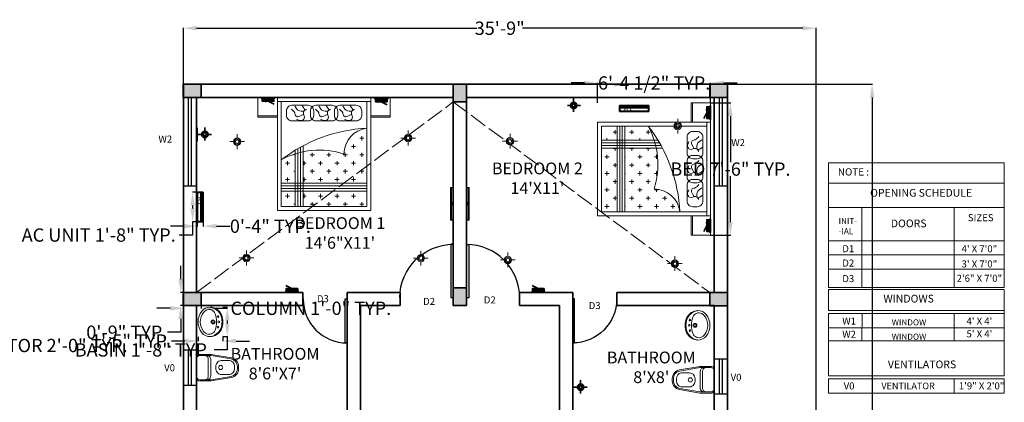
# Model space of a CAD drawing. Units: inches. Extents: x 68 to 1275, y 90 to 1276.
# Tile 6 of 6: x 608 to 1275, y 1017 to 1276. Entities that reach past the tile are written whole.
import ezdxf

# ---------------------------------------------------------------- set-up
doc = ezdxf.new("R2010")
doc.units = ezdxf.units.IN
doc.header["$MEASUREMENT"] = 0
doc.linetypes.add('ACAD_ISO02W100', pattern=[15, 12, -3])
for name, color, linetype, lineweight in [('A -Elec', 6, 'Continuous', 18), ('A-ANNO-SCHD', 8, 'Continuous', 13), ('A-ANNO-TEXT', 7, 'Continuous', 18), ('A-AREA-IDEN', 7, 'Continuous', 18), ('A-FLOR-FIXT', 9, 'Continuous', 18), ('A-FURN', 150, 'Continuous', 5), ('A-WALL', 7, 'Continuous', 35), ('COLUMN', 150, 'Continuous', 35), ('DIM', 2, 'Continuous', 18), ('DOOR', 15, 'Continuous', 25), ('E-EQPM', 1, 'Continuous', 18), ('E-LITE', 6, 'Continuous', 18), ('E-POWR', 1, 'Continuous', 18), ('E-REFR', 8, 'ACAD_ISO02W100', 13), ('Elec', 1, 'Continuous', 35), ('FURN', 163, 'Continuous', 18), ('WINDOW', 17, 'Continuous', 18)]:
    doc.layers.add(name, color=color, linetype=linetype, lineweight=lineweight)
doc.styles.get("Standard").update_dxf_attribs({"font": 'arial.ttf'})
doc.dimstyles.get("Standard").update_dxf_attribs({"dimtxt": 9, "dimasz": 9, "dimexe": 0.18, "dimexo": 0.0625, "dimgap": 0.09, "dimtad": 0, "dimtih": 1, "dimtoh": 1, "dimdec": 1, "dimzin": 0, "dimdsep": 46, "dimlunit": 3, "dimtxsty": 'Standard', "dimcen": 0.09, "dimadec": 0, "dimazin": 0, "dimtfac": 1, "dimtdec": 1, "dimtofl": 0, "dimtmove": 0, "dimatfit": 3, "dimfxl": 1, "dimtolj": 1, "dimtzin": 0, "dimarcsym": 0})

# ---------------------------------------------------------------- blocks, each defined once
blk = doc.blocks.new('*U2')
for p, q in [((0, 0), (0, -6)), ((40, 0), (40, -6))]:
    blk.add_line(p, q)
blk.add_lwpolyline([(0, 0), (0, 40), (1.75, 40), (1.75, 0)], close=True)
blk.add_arc((0, 0), 40, 0, 90)
blk = doc.blocks.new('W')
at = {"layer": 'DOOR'}
for p, q in [((91.84, 414.95), (100.84, 414.95)), ((91.84, 354.95), (91.84, 414.95)), ((95.34, 354.95), (95.34, 414.95)), ((97.34, 354.95), (97.34, 414.95)), ((100.84, 414.95), (100.84, 354.95)), ((100.84, 354.95), (91.84, 354.95))]:
    blk.add_line(p, q, dxfattribs=at)
blk = doc.blocks.new('V')
at = {"layer": 'DOOR'}
for p, q in [((554.81, 674.59), (563.81, 674.59)), ((554.81, 650.59), (554.81, 674.59)), ((558.31, 650.59), (558.31, 674.59)), ((560.31, 650.59), (560.31, 674.59)), ((563.81, 674.59), (563.81, 650.59)), ((563.81, 650.59), (554.81, 650.59))]:
    blk.add_line(p, q, dxfattribs=at)
blk = doc.blocks.new('C')
h = blk.add_hatch(color=256)
h.dxf.hatch_style = 1
h.paths.add_polyline_path([(745.81, 845.98), (745.81, 857.98), (736.81, 857.98), (736.81, 845.98)])
for p, q in [((745.81, 857.98), (736.81, 857.98)), ((736.81, 857.98), (736.81, 845.98)), ((745.81, 845.98), (745.81, 857.98)), ((736.81, 845.98), (745.81, 845.98))]:
    blk.add_line(p, q)
blk = doc.blocks.new('bed 1')
at = {"layer": 'FURN'}
h = blk.add_hatch(dxfattribs=at)
h.set_pattern_fill('CROSS', color=256, style=0)
h.set_pattern_definition([(0, (0, 0), (6.35, 6.35), [3.175, -9.525]), (90, (1.5875, -1.5875), (-6.35, 6.35), [3.175, -9.525])])
h.paths.add_polyline_path([(1334.16, -843.32, 0.37496), (1316.43, -863.27, 0.131129), (1284.95, -861.51), (1284.95, -885.72), (1334.16, -885.72)])
h.paths.add_polyline_path([(1278.95, -863.08, 0.048033), (1268.16, -867.67), (1268.16, -885.72), (1278.95, -885.72)])
h.paths.add_polyline_path([(1278.95, -891.72), (1268.16, -891.72), (1268.16, -903.72), (1278.95, -903.72)])
h.paths.add_polyline_path([(1334.16, -891.72), (1284.95, -891.72), (1284.95, -903.72), (1334.16, -903.72)])
for p, q in [((1265.16, -819.72), (1250.16, -819.72)), ((1250.16, -819.72), (1250.16, -834.72)), ((1337.16, -819.72), (1265.16, -819.72)), ((1265.16, -819.72), (1265.16, -906.72)), ((1337.16, -822.72), (1265.16, -822.72)), ((1268.16, -822.72), (1268.16, -903.72)), ((1334.16, -903.72), (1334.16, -822.72)), ((1337.16, -906.72), (1337.16, -819.72)), ((1337.16, -819.72), (1352.16, -819.72)), ((1352.16, -819.72), (1352.16, -834.72)), ((1250.16, -833.72), (1265.16, -833.72)), ((1352.16, -833.72), (1337.16, -833.72)), ((1250.16, -834.72), (1265.16, -834.72)), ((1352.16, -834.72), (1337.16, -834.72)), ((1284.95, -903.72), (1284.95, -856.89)), ((1278.95, -903.72), (1278.95, -860.29)), ((1280.95, -903.72), (1280.95, -859.11)), ((1282.95, -903.72), (1282.95, -857.98)), ((1334.16, -885.72), (1268.16, -885.72)), ((1334.16, -887.72), (1268.16, -887.72)), ((1334.16, -889.72), (1268.16, -889.72)), ((1334.16, -891.72), (1268.16, -891.72)), ((1265.16, -906.72), (1337.16, -906.72)), ((1268.16, -903.72), (1334.16, -903.72))]:
    blk.add_line(p, q, dxfattribs=at)
for points in [[(1288.91, -837.72), (1276.42, -837.72, -0.414214), (1272.16, -833.47), (1272.16, -829.98, -0.414214), (1276.42, -825.72), (1288.91, -825.72, -0.414214), (1293.16, -829.98), (1293.16, -833.47, -0.414214)], [(1307.41, -837.72), (1294.92, -837.72, -0.414214), (1290.66, -833.47), (1290.66, -829.98, -0.414214), (1294.92, -825.72), (1307.41, -825.72, -0.414214), (1311.66, -829.98), (1311.66, -833.47, -0.414214)], [(1325.91, -837.72), (1313.42, -837.72, -0.414214), (1309.16, -833.47), (1309.16, -829.98, -0.414214), (1313.42, -825.72), (1325.91, -825.72, -0.414214), (1330.16, -829.98), (1330.16, -833.47, -0.414214)], [(1334.16, -843.32, 0.151933), (1268.16, -867.67), (1268.16, -867.67, -0.20661), (1316.43, -863.27), (1316.43, -863.27, -0.37496)]]:
    blk.add_lwpolyline(points, format="xyb", close=True, dxfattribs=at)
for points, knots in [([(1278.62, -826.37), (1279.52, -827.92), (1281.07, -830.61), (1287.77, -830.3), (1285.41, -827.44), (1284.17, -825.93)], [0, 0, 0, 0, 4.23607, 7.317462, 10.761159, 10.761159, 10.761159, 10.761159]), ([(1297.12, -826.37), (1298.02, -827.92), (1299.57, -830.61), (1306.27, -830.3), (1303.91, -827.44), (1302.67, -825.93)], [0, 0, 0, 0, 4.23607, 7.317462, 10.761159, 10.761159, 10.761159, 10.761159]), ([(1315.62, -826.37), (1316.52, -827.92), (1318.07, -830.61), (1324.77, -830.3), (1322.41, -827.44), (1321.17, -825.93)], [0, 0, 0, 0, 4.23607, 7.317462, 10.761159, 10.761159, 10.761159, 10.761159]), ([(1275.98, -828.74), (1277, -829.54), (1278.71, -830.85), (1279.22, -835.95), (1282.92, -833.91), (1285.58, -832.44)], [0, 0, 0, 0, 3.079719, 5.108686, 10.317752, 10.317752, 10.317752, 10.317752]), ([(1287.7, -828.74), (1286.63, -829.38), (1283.96, -830.98), (1287.28, -835.52), (1283.18, -838.02), (1281.17, -836.99), (1280.03, -836.4)], [0, 0, 0, 0, 2.624379, 6.568207, 8.823918, 11.783788, 11.783788, 11.783788, 11.783788]), ([(1294.48, -828.74), (1295.5, -829.54), (1297.21, -830.85), (1297.72, -835.95), (1301.42, -833.91), (1304.08, -832.44)], [0, 0, 0, 0, 3.079719, 5.108686, 10.317752, 10.317752, 10.317752, 10.317752]), ([(1306.2, -828.74), (1305.13, -829.38), (1302.46, -830.98), (1305.78, -835.52), (1301.68, -838.02), (1299.67, -836.99), (1298.53, -836.4)], [0, 0, 0, 0, 2.624379, 6.568207, 8.823918, 11.783788, 11.783788, 11.783788, 11.783788]), ([(1312.98, -828.74), (1314, -829.54), (1315.71, -830.85), (1316.22, -835.95), (1319.92, -833.91), (1322.58, -832.44)], [0, 0, 0, 0, 3.079719, 5.108686, 10.317752, 10.317752, 10.317752, 10.317752]), ([(1324.7, -828.74), (1323.63, -829.38), (1320.96, -830.98), (1324.28, -835.52), (1320.18, -838.02), (1318.17, -836.99), (1317.03, -836.4)], [0, 0, 0, 0, 2.624379, 6.568207, 8.823918, 11.783788, 11.783788, 11.783788, 11.783788])]:
    blk.add_open_spline(points, degree=3, knots=knots, dxfattribs=at)
blk = doc.blocks.new('WC')
at = {"layer": 'A-FURN'}
for p, q in [((171114.18, -56009.21), (171100.52, -56011.54)), ((171114.18, -56009.21), (171122.29, -56009.21)), ((171124.07, -56010.99), (171124.07, -56025.42)), ((171095.59, -56017.39), (171095.59, -56019.02)), ((171114.18, -56027.21), (171100.52, -56024.87)), ((171122.29, -56027.21), (171114.18, -56027.21))]:
    blk.add_line(p, q, dxfattribs=at)
for points in [[(171114.18, -56027.21), (171122.29, -56027.21, 0.414214), (171124.07, -56025.42), (171124.07, -56010.99, 0.414214), (171122.29, -56009.21), (171114.18, -56009.21), (171100.52, -56011.54, 0.365402), (171095.59, -56017.39), (171095.59, -56019.02, 0.365402), (171100.52, -56024.87)], [(171114.25, -56026.41), (171121.5, -56026.41, 0.361508), (171124.07, -56024.7), (171124.07, -56011.71, 0.375474), (171121.68, -56010), (171114.25, -56010), (171100.66, -56012.32, 0.365402), (171096.38, -56017.39), (171096.38, -56019.02, 0.365402), (171100.66, -56024.09)], [(171106.42, -56023.02, 0.46477), (171111.04, -56019.12), (171111.04, -56017.49, 0.46477), (171106.42, -56013.59), (171101.64, -56013.59, 0.365402), (171098.35, -56017.49), (171098.35, -56019.12, 0.365402), (171101.64, -56023.02)], [(171124.07, -56011.71), (171124.07, -56024.7, -0.361508), (171121.5, -56026.41), (171117.23, -56026.41, -0.430105), (171114.38, -56023.46), (171114.38, -56012.95, -0.411531), (171117.23, -56010), (171121.68, -56010, -0.375474)], [(171124.07, -56011.71), (171124.07, -56024.7, -0.361508), (171121.5, -56026.41), (171118.83, -56026.41, -0.480412), (171116.16, -56023.63), (171116.16, -56012.78, -0.482705), (171118.83, -56010), (171121.68, -56010, -0.375474)], [(171107.8, -56016.9, -1), (171107.8, -56019.71, -1)]]:
    blk.add_lwpolyline(points, format="xyb", close=True, dxfattribs=at)
for centre, radius, start, end in [((171101.52, -56017.39), 5.93, 99.71057, 180.00015), ((171122.29, -56010.99), 1.78, 0.00015, 90.00015), ((171101.52, -56019.02), 5.93, 180.00015, 260.28974), ((171122.29, -56025.42), 1.78, 270.00015, 0.00015)]:
    blk.add_arc(centre, radius, start, end, dxfattribs=at)
blk = doc.blocks.new('Basin')
at = {"layer": 'A-FURN'}
for centre, radius in [((171010.45, -56072.47), 0.692), ((171010.96, -56068.51), 0.593), ((171014.68, -56072.47), 1.48), ((171014.68, -56072.47), 0.91), ((171010.96, -56076.42), 0.593)]:
    blk.add_circle(centre, radius, dxfattribs=at)
for centre, radius, start, end in [((171018.29, -56073.43), 10.2, 262.50469, 262.50469), ((171016.96, -56070.69), 9.3, 90, 157.28559), ((171018.29, -56071.51), 10.2, 100.99675, 157.82074), ((171029.84, -56072.47), 17.8, 159.64154, 180), ((171017.65, -56067.95), 4.81, 62.93101, 159.64154), ((171016.96, -56069.3), 7.91, 39.08291, 90), ((171016.96, -56069.3), 6.33, 39.08291, 62.931), ((171013.06, -56072.47), 11.35, 0, 39.08291), ((171013.06, -56072.47), 12.93, 0, 39.08291), ((171021.21, -56072.47), 13.91, 157.28559, 180), ((171021.21, -56072.47), 13.91, 180, 202.71441), ((171021.21, -56072.47), 13.27, 158.74675, 180), ((171021.21, -56072.47), 13.27, 180, 201.25325), ((171029.84, -56072.47), 17.8, 180, 200.35846), ((171013.06, -56072.47), 11.35, 320.91709, 0), ((171013.06, -56072.47), 12.93, 320.91709, 0), ((171016.96, -56074.25), 9.3, 202.71441, 270), ((171018.29, -56073.43), 10.2, 202.17926, 259.00325), ((171017.65, -56076.99), 4.81, 200.35846, 297.06899), ((171016.96, -56075.63), 7.91, 270, 320.91709), ((171016.96, -56075.63), 6.33, 297.069, 320.91709)]:
    blk.add_arc(centre, radius, start, end, dxfattribs=at)
blk = doc.blocks.new('splight')
at = {"layer": 'Elec'}
for p, q in [((4620.58, 521.58), (4618.05, 521.58)), ((4618.17, 527.16), (4627.57, 527.16)), ((4622.87, 527.16), (4622.87, 523.87)), ((4625.16, 521.58), (4627.23, 521.58)), ((4622.87, 519.28), (4622.87, 517.03))]:
    blk.add_line(p, q, dxfattribs=at)
for radius in [2.29, 1.67, 1.04]:
    blk.add_circle((4622.87, 521.58), radius, dxfattribs=at)
blk = doc.blocks.new('tube')
at = {"layer": 'A -Elec'}
for p, q in [((4592.6, 556.8), (4641.6, 556.8)), ((4592.6, 555.3), (4592.6, 556.8)), ((4592.6, 552.8), (4592.6, 555.3)), ((4592.6, 552.8), (4641.6, 552.8)), ((4593.1, 555.3), (4593.1, 556.8)), ((4593.1, 556.3), (4593.4, 556.3)), ((4593.1, 556.2), (4593.4, 556.2)), ((4593.1, 555.8), (4593.4, 555.8)), ((4593.1, 555.7), (4593.4, 555.7)), ((4641.1, 555.3), (4593.1, 555.3)), ((4593.1, 555.3), (4593.1, 553.3)), ((4593.1, 553.3), (4593.1, 555.3)), ((4593.1, 553.3), (4641.6, 553.3)), ((4593.4, 555.3), (4593.4, 556.8)), ((4593.4, 556.5), (4640.8, 556.5)), ((4593.4, 556.3), (4640.8, 556.3)), ((4593.4, 556), (4640.8, 556)), ((4593.4, 555.8), (4640.8, 555.8)), ((4593.4, 555.5), (4640.8, 555.5)), ((4640.8, 555.3), (4640.8, 556.8)), ((4640.8, 556.3), (4641.1, 556.3)), ((4640.8, 556.2), (4641.1, 556.2)), ((4640.8, 555.8), (4641.1, 555.8)), ((4640.8, 555.7), (4641.1, 555.7)), ((4641.1, 556.8), (4641.1, 555.3)), ((4641.1, 555.3), (4641.1, 556.8)), ((4641.1, 553.3), (4641.1, 555.3)), ((4641.6, 556.8), (4641.6, 555.3)), ((4641.6, 552.8), (4641.6, 555.3))]:
    blk.add_line(p, q, dxfattribs=at)
for points in [[(4615.6, 553.3), (4619.1, 553.3), (4619.1, 554.3), (4615.6, 554.3)], [(4619.1, 553.8), (4619.1, 553.8), (4619.1, 553.8), (4619.1, 553.8)], [(4619.1, 553.8), (4619.8, 553.8), (4619.8, 553.3), (4619.1, 553.3)]]:
    blk.add_lwpolyline(points, close=True, dxfattribs=at)
blk = doc.blocks.new('CIELING')
at = {"layer": 'A -Elec'}
for p, q in [((1070.9, -8395.7), (1070.9, -8391.5)), ((1066.6, -8399.9), (1062.4, -8399.9)), ((1070.9, -8408.3), (1070.9, -8404.2)), ((1075.1, -8399.9), (1079.3, -8399.9))]:
    blk.add_line(p, q, dxfattribs=at)
for radius in [4.26, 3.1, 1.94]:
    blk.add_circle((1070.9, -8399.9), radius, dxfattribs=at)
blk = doc.blocks.new('ac')
at = {"layer": 'Elec'}
for p, q in [((12718.3, -53.8), (12674.4, -53.8)), ((12674.4, -63), (12674.4, -53.8)), ((12674.9, -57.5), (12717.8, -57.5)), ((12675.8, -57.5), (12675.8, -53.8)), ((12717, -54.9), (12675.8, -54.9)), ((12717, -56.2), (12675.8, -56.2)), ((12717, -57.5), (12717, -53.8)), ((12718.3, -63), (12718.3, -53.8)), ((12718.3, -63), (12674.4, -63))]:
    blk.add_line(p, q, dxfattribs=at)
at = {"layer": 'Elec', "ltscale": 0.1}
for p, q in [((12674.9, -61.5), (12674.9, -53.8)), ((12717, -54.4), (12675.8, -54.4)), ((12717, -55.7), (12675.8, -55.7)), ((12717, -56.8), (12675.8, -56.8)), ((12717.8, -61.5), (12717.8, -53.8)), ((12716.8, -62.5), (12675.9, -62.5))]:
    blk.add_line(p, q, dxfattribs=at)
at = {"layer": 'Elec'}
for centre, start, end in [((12675.9, -61.5), 180, 270), ((12716.8, -61.5), 270, 0)]:
    blk.add_arc(centre, 1, start, end, dxfattribs=at)
blk = doc.blocks.new('elec box')
at = {"layer": 'Elec'}
blk.add_hatch(color=256, dxfattribs=at).paths.add_polyline_path([(3828.2, 599.3), (3828.2, 594.8), (3844.7, 594.8), (3844.7, 599.3)])
for p, q in [((3836.5, 599.3), (3828.1, 603.5)), ((3846.1, 594.8), (3826.8, 594.8)), ((3826.8, 594.8), (3826.8, 593.9)), ((3826.8, 593.9), (3846.1, 593.9)), ((3846.1, 593.9), (3846.1, 594.8))]:
    blk.add_line(p, q, dxfattribs=at)
blk.add_lwpolyline([(3828.2, 594.8), (3828.2, 599.3), (3844.7, 599.3), (3844.7, 594.8), (3828.2, 594.8)], dxfattribs=at)
blk = doc.blocks.new('SWITCHBOARD-ONE-WAY')
blk.add_line((4.63, 1.73), (6.64, 3.12))
at = {"xscale": 0.480395109260985, "yscale": 0.480395109260985, "zscale": 0.480395109260985}
blk.add_blockref('elec box', (-1838.39, -285.3), dxfattribs=at)
blk = doc.blocks.new('SWITCHBOARD-TWO-WAY')
for q in [(2.61, 1.47), (6.62, 1.46)]:
    blk.add_line((4.62, 2.87), q)
at = {"xscale": 0.480395109260985, "yscale": 0.480395109260985, "zscale": 0.480395109260985, "rotation": 180}
blk.add_blockref('elec box', (1847.65, 289.9), dxfattribs=at)
blk = doc.blocks.new('*D49')
at = {"layer": 'Defpoints', "color": 0, "transparency": 16777216}
for p in [(534.19, 1046.47), (537.79, 1046.47), (534.19, 1022.47)]:
    blk.add_point(p, dxfattribs=at)
at = {"layer": 'DIM', "color": 0, "lineweight": -2, "transparency": 16777216}
for p, q in [((537.79, 1046.47), (537.79, 1055.47)), ((537.79, 1055.47), (546.79, 1055.47)), ((534.25, 1046.47), (537.97, 1046.47)), ((537.79, 1031.47), (537.79, 1037.47)), ((534.25, 1022.47), (537.97, 1022.47))]:
    blk.add_line(p, q, dxfattribs=at)
at = {"layer": 'DIM', "color": 0, "transparency": 16777216}
for points in [[(536.29, 1037.47), (539.29, 1037.47), (537.79, 1046.47)], [(536.29, 1031.47), (539.29, 1031.47), (537.79, 1022.47)]]:
    blk.add_solid(points, dxfattribs=at)
at = {"layer": 'DIM', "color": 0, "transparency": 16777216, "insert": (615.76, 1055.47), "char_height": 9, "attachment_point": 5}
blk.add_mtext('\\A1;VENTILATOR 2\'-0" TYP.', dxfattribs=at)
blk = doc.blocks.new('*D55')
at = {"layer": 'Defpoints', "color": 0, "transparency": 16777216}
for p in [(1076.08, 1219.88), (1076.08, 1130.12), (1089.54, 1130.12)]:
    blk.add_point(p, dxfattribs=at)
at = {"layer": 'DIM', "color": 0, "lineweight": -2, "transparency": 16777216}
for p, q in [((1076.14, 1219.88), (1089.72, 1219.88)), ((1089.54, 1210.88), (1089.54, 1179.68)), ((1089.54, 1139.12), (1089.54, 1170.31)), ((1076.14, 1130.12), (1089.72, 1130.12))]:
    blk.add_line(p, q, dxfattribs=at)
at = {"layer": 'DIM', "color": 0, "transparency": 16777216}
for points in [[(1088.04, 1210.88), (1091.04, 1210.88), (1089.54, 1219.88)], [(1088.04, 1139.12), (1091.04, 1139.12), (1089.54, 1130.12)]]:
    blk.add_solid(points, dxfattribs=at)
at = {"layer": 'DIM', "color": 0, "transparency": 16777216, "insert": (1089.54, 1175), "char_height": 9, "attachment_point": 5}
blk.add_mtext('\\A1;BED 7\'-6" TYP.', dxfattribs=at)
blk = doc.blocks.new('*D56')
at = {"layer": 'Defpoints', "color": 0, "transparency": 16777216}
for p in [(1076.08, 1233.34), (999.52, 1219.88), (1076.08, 1219.88)]:
    blk.add_point(p, dxfattribs=at)
at = {"layer": 'DIM', "color": 0, "lineweight": -2, "transparency": 16777216}
for p, q in [((990.52, 1233.34), (981.52, 1233.34)), ((999.52, 1219.94), (999.52, 1233.52)), ((1076.08, 1219.94), (1076.08, 1233.52)), ((1085.08, 1233.34), (1094.08, 1233.34))]:
    blk.add_line(p, q, dxfattribs=at)
at = {"layer": 'DIM', "color": 0, "transparency": 16777216}
for points in [[(990.52, 1234.84), (990.52, 1231.84), (999.52, 1233.34)], [(1085.08, 1234.84), (1085.08, 1231.84), (1076.08, 1233.34)]]:
    blk.add_solid(points, dxfattribs=at)
at = {"layer": 'DIM', "color": 0, "transparency": 16777216, "insert": (1037.8, 1233.34), "char_height": 9, "attachment_point": 5}
blk.add_mtext('\\A1;6\'-4 1/2" TYP.', dxfattribs=at)
blk = doc.blocks.new('*D57')
at = {"layer": 'Defpoints', "color": 0, "transparency": 16777216}
for p in [(718.63, 1082.48), (730.63, 1082.48), (730.63, 1080.68)]:
    blk.add_point(p, dxfattribs=at)
at = {"layer": 'DIM', "color": 0, "lineweight": -2, "transparency": 16777216}
for p, q in [((718.63, 1082.42), (718.63, 1080.5)), ((730.63, 1082.42), (730.63, 1080.5)), ((709.63, 1080.68), (700.63, 1080.68)), ((739.63, 1080.68), (748.63, 1080.68))]:
    blk.add_line(p, q, dxfattribs=at)
at = {"layer": 'DIM', "color": 0, "transparency": 16777216}
for points in [[(709.63, 1082.18), (709.63, 1079.18), (718.63, 1080.68)], [(739.63, 1082.18), (739.63, 1079.18), (730.63, 1080.68)]]:
    blk.add_solid(points, dxfattribs=at)
at = {"layer": 'DIM', "color": 0, "transparency": 16777216, "insert": (805.08, 1080.68), "char_height": 9, "attachment_point": 5}
blk.add_mtext('\\A1;COLUMN 1\'-0" TYP.', dxfattribs=at)
blk = doc.blocks.new('*D58')
at = {"layer": 'Defpoints', "color": 0, "transparency": 16777216}
for p in [(718.63, 1091.48), (716.83, 1082.48), (718.63, 1082.48)]:
    blk.add_point(p, dxfattribs=at)
at = {"layer": 'DIM', "color": 0, "lineweight": -2, "transparency": 16777216}
for p, q in [((716.83, 1100.48), (716.83, 1109.48)), ((718.56, 1091.48), (716.65, 1091.48)), ((718.56, 1082.48), (716.65, 1082.48)), ((716.83, 1073.48), (716.83, 1064.48)), ((716.83, 1064.48), (707.83, 1064.48))]:
    blk.add_line(p, q, dxfattribs=at)
at = {"layer": 'DIM', "color": 0, "transparency": 16777216}
for points in [[(715.33, 1100.48), (718.33, 1100.48), (716.83, 1091.48)], [(715.33, 1073.48), (718.33, 1073.48), (716.83, 1082.48)]]:
    blk.add_solid(points, dxfattribs=at)
at = {"layer": 'DIM', "color": 0, "transparency": 16777216, "insert": (680.31, 1064.48), "char_height": 9, "attachment_point": 5}
blk.add_mtext('\\A1;0\'-9" TYP.', dxfattribs=at)
blk = doc.blocks.new('*D61')
at = {"layer": 'Defpoints', "color": 0, "transparency": 16777216}
for p in [(745.43, 1081.42), (745.43, 1061.49), (748.42, 1061.49)]:
    blk.add_point(p, dxfattribs=at)
at = {"layer": 'DIM', "color": 0, "lineweight": -2, "transparency": 16777216}
for p, q in [((745.49, 1081.42), (748.6, 1081.42)), ((748.42, 1072.42), (748.42, 1070.49)), ((745.49, 1061.49), (748.6, 1061.49)), ((748.42, 1061.49), (748.42, 1052.49)), ((748.42, 1052.49), (739.42, 1052.49))]:
    blk.add_line(p, q, dxfattribs=at)
at = {"layer": 'DIM', "color": 0, "transparency": 16777216}
for points in [[(746.92, 1072.42), (749.92, 1072.42), (748.42, 1081.42)], [(746.92, 1070.49), (749.92, 1070.49), (748.42, 1061.49)]]:
    blk.add_solid(points, dxfattribs=at)
at = {"layer": 'DIM', "color": 0, "transparency": 16777216, "insert": (691.48, 1052.49), "char_height": 9, "attachment_point": 5}
blk.add_mtext('\\A1;BASIN 1\'-8" TYP.', dxfattribs=at)
blk = doc.blocks.new('*D62')
at = {"layer": 'Defpoints', "color": 0, "transparency": 16777216}
for p in [(728.6, 1061.49), (745.43, 1061.49), (728.6, 1058.5)]:
    blk.add_point(p, dxfattribs=at)
at = {"layer": 'DIM', "color": 0, "lineweight": -2, "transparency": 16777216}
for p, q in [((728.6, 1061.42), (728.6, 1058.32)), ((745.43, 1061.42), (745.43, 1058.32)), ((719.6, 1058.5), (710.6, 1058.5)), ((754.43, 1058.5), (763.43, 1058.5))]:
    blk.add_line(p, q, dxfattribs=at)
at = {"layer": 'DIM', "color": 0, "transparency": 16777216}
for points in [[(719.6, 1060), (719.6, 1057), (728.6, 1058.5)], [(754.43, 1060), (754.43, 1057), (745.43, 1058.5)]]:
    blk.add_solid(points, dxfattribs=at)
at = {"layer": 'DIM', "color": 0, "transparency": 16777216, "insert": (683.51, 1058.5), "char_height": 9, "attachment_point": 5}
blk.add_mtext('\\A1;1\'-5" TYP.', dxfattribs=at)
blk = doc.blocks.new('*D73')
at = {"layer": 'Defpoints', "color": 0, "transparency": 16777216}
for p in [(727.92, 1159.31), (724.91, 1139.3), (727.92, 1139.3)]:
    blk.add_point(p, dxfattribs=at)
at = {"layer": 'DIM', "color": 0, "lineweight": -2, "transparency": 16777216}
for p, q in [((727.85, 1159.31), (724.73, 1159.31)), ((724.91, 1150.31), (724.91, 1148.3)), ((727.85, 1139.3), (724.73, 1139.3)), ((724.91, 1139.3), (724.91, 1130.3)), ((724.91, 1130.3), (715.91, 1130.3))]:
    blk.add_line(p, q, dxfattribs=at)
at = {"layer": 'DIM', "color": 0, "transparency": 16777216}
for points in [[(723.41, 1150.31), (726.41, 1150.31), (724.91, 1159.31)], [(723.41, 1148.3), (726.41, 1148.3), (724.91, 1139.3)]]:
    blk.add_solid(points, dxfattribs=at)
at = {"layer": 'DIM', "color": 0, "transparency": 16777216, "insert": (661.24, 1130.3), "char_height": 9, "attachment_point": 5}
blk.add_mtext('\\A1;AC UNIT 1\'-8" TYP.', dxfattribs=at)
blk = doc.blocks.new('*D74')
at = {"layer": 'Defpoints', "color": 0, "transparency": 16777216}
for p in [(727.92, 1139.3), (732.12, 1139.3), (732.12, 1136.3)]:
    blk.add_point(p, dxfattribs=at)
at = {"layer": 'DIM', "color": 0, "lineweight": -2, "transparency": 16777216}
for p, q in [((718.92, 1136.3), (709.92, 1136.3)), ((727.92, 1139.24), (727.92, 1136.12)), ((732.12, 1139.24), (732.12, 1136.12)), ((741.12, 1136.3), (750.12, 1136.3))]:
    blk.add_line(p, q, dxfattribs=at)
at = {"layer": 'DIM', "color": 0, "transparency": 16777216}
for points in [[(718.92, 1137.8), (718.92, 1134.8), (727.92, 1136.3)], [(741.12, 1137.8), (741.12, 1134.8), (732.12, 1136.3)]]:
    blk.add_solid(points, dxfattribs=at)
at = {"layer": 'DIM', "color": 0, "transparency": 16777216, "insert": (777.64, 1136.3), "char_height": 9, "attachment_point": 5}
blk.add_mtext('\\A1;0\'-4" TYP.', dxfattribs=at)
blk = doc.blocks.new('*D112')
at = {"layer": 'Defpoints', "color": 0, "transparency": 16777216}
for p in [(1147.63, 1270.42), (718.63, 1232.47), (1147.63, 988.68)]:
    blk.add_point(p, dxfattribs=at)
at = {"layer": 'DIM', "color": 0, "lineweight": -2, "transparency": 16777216}
for p, q in [((718.63, 1232.53), (718.63, 1270.6)), ((727.63, 1270.42), (917.58, 1270.42)), ((1138.63, 1270.42), (948.67, 1270.42)), ((1147.63, 988.74), (1147.63, 1270.6))]:
    blk.add_line(p, q, dxfattribs=at)
at = {"layer": 'DIM', "color": 0, "transparency": 16777216}
for points in [[(727.63, 1271.92), (727.63, 1268.92), (718.63, 1270.42)], [(1138.63, 1271.92), (1138.63, 1268.92), (1147.63, 1270.42)]]:
    blk.add_solid(points, dxfattribs=at)
at = {"layer": 'DIM', "color": 0, "transparency": 16777216, "insert": (933.13, 1270.42), "char_height": 9, "attachment_point": 5}
blk.add_mtext('\\A1;35\'-9"', dxfattribs=at)
blk = doc.blocks.new('*D113')
at = {"layer": 'Defpoints', "color": 0, "transparency": 16777216}
for p in [(1087.63, 1232.47), (1185.58, 1232.47), (1087.63, 603.47)]:
    blk.add_point(p, dxfattribs=at)
at = {"layer": 'DIM', "color": 0, "lineweight": -2, "transparency": 16777216}
for p, q in [((1087.69, 1232.47), (1185.76, 1232.47)), ((1185.58, 1223.47), (1185.58, 922.65)), ((1185.58, 612.47), (1185.58, 913.28)), ((1087.69, 603.47), (1185.76, 603.47))]:
    blk.add_line(p, q, dxfattribs=at)
at = {"layer": 'DIM', "color": 0, "transparency": 16777216}
for points in [[(1184.08, 1223.47), (1187.08, 1223.47), (1185.58, 1232.47)], [(1184.08, 612.47), (1187.08, 612.47), (1185.58, 603.47)]]:
    blk.add_solid(points, dxfattribs=at)
at = {"layer": 'DIM', "color": 0, "transparency": 16777216, "insert": (1185.58, 917.97), "char_height": 9, "attachment_point": 5}
blk.add_mtext('\\A1;52\'-5"', dxfattribs=at)

msp = doc.modelspace()

# ---------------------------------------------------------------- linework, layer by layer
at = {"layer": 'A-ANNO-SCHD'}
for p, q in [((1155.94, 1179.2), (1155.94, 1107.08)), ((1155.94, 1165.48), (1275.19, 1165.48)), ((1155.94, 1149.03), (1275.19, 1149.03)), ((1178.72, 1126.49), (1178.72, 1149.03)), ((1241.26, 1126.49), (1241.26, 1149.03)), ((1155.94, 1126.49), (1275.19, 1126.49)), ((1178.72, 1094.8), (1178.72, 1126.49)), ((1241.26, 1094.8), (1241.26, 1126.49)), ((1155.94, 1116.79), (1275.19, 1116.79)), ((1155.94, 1107.08), (1275.19, 1107.08)), ((1155.94, 1107.08), (1155.94, 1094.8)), ((1275.19, 1094.8), (1275.19, 1106.77)), ((1155.94, 1094.8), (1275.19, 1094.8)), ((1275.19, 1077.18), (1275.19, 1093.33)), ((1178.74, 1058.74), (1178.75, 1077.18)), ((1241.26, 1058.74), (1241.26, 1077.18)), ((1155.97, 1067.47), (1275.23, 1067.47)), ((1155.94, 1058.74), (1275.19, 1058.74)), ((1241.26, 1023.23), (1241.26, 1032.94))]:
    msp.add_line(p, q, dxfattribs=at)
for points in [[(1155.94, 1179.2), (1275.19, 1179.2), (1275.19, 1106.77)], [(1275.19, 1079.24), (1155.94, 1079.24), (1155.94, 1093.33), (1275.19, 1093.33)], [(1155.94, 1058.74), (1155.94, 1077.18), (1275.19, 1077.18), (1275.19, 1058.74)], [(1275.19, 1023.23), (1155.94, 1023.23), (1155.94, 1032.94), (1275.19, 1032.94)], [(1275.19, 1032.94), (1275.19, 1023.23), (1158.16, 1023.23)]]:
    msp.add_lwpolyline(points, dxfattribs=at)
msp.add_lwpolyline([(1275.19, 1034.99), (1155.94, 1034.99), (1155.94, 1058.74), (1275.19, 1058.74), (1275.19, 1034.99)], close=True, dxfattribs=at)
at = {"layer": 'A-WALL'}
for p, q in [((718.63, 1232.47), (1087.63, 1232.47)), ((718.63, 1232.47), (718.63, 603.47)), ((1087.63, 1232.47), (1087.63, 977.47)), ((727.63, 1223.47), (718.63, 1223.47)), ((727.63, 1223.47), (901.63, 1223.47)), ((727.63, 1223.47), (727.63, 1091.47)), ((901.63, 1223.47), (901.63, 1091.47)), ((910.63, 1223.47), (1078.63, 1223.47)), ((910.63, 1223.47), (910.63, 1091.47)), ((1078.63, 1223.47), (1078.63, 1091.47)), ((1078.63, 1223.47), (1087.63, 1223.47)), ((901.63, 1220.47), (910.63, 1220.47)), ((727.63, 1091.47), (799.63, 1091.47)), ((799.63, 1082.47), (799.63, 1091.47)), ((829.63, 1091.47), (865.63, 1091.47)), ((829.63, 1082.47), (829.63, 1091.47)), ((865.63, 1091.47), (865.63, 1082.47)), ((901.63, 1091.47), (901.63, 1082.47)), ((910.63, 1091.47), (910.63, 1082.47)), ((946.63, 1091.47), (982.63, 1091.47)), ((946.63, 1091.47), (946.63, 1082.47)), ((982.63, 1082.47), (982.63, 1091.47)), ((1012.63, 1091.47), (1078.63, 1091.47)), ((1012.63, 1082.47), (1012.63, 1091.47)), ((727.63, 1082.47), (799.63, 1082.47)), ((727.63, 1082.47), (727.63, 998.47)), ((829.63, 1082.47), (829.63, 998.47)), ((838.63, 1082.47), (865.63, 1082.47)), ((838.63, 1082.47), (838.63, 986.47)), ((901.63, 1082.47), (910.63, 1082.47)), ((946.63, 1082.47), (973.63, 1082.47)), ((973.63, 1082.47), (973.63, 977.47)), ((982.63, 1082.47), (982.63, 986.47)), ((1012.63, 1082.47), (1078.63, 1082.47)), ((1078.63, 1082.47), (1078.63, 986.47))]:
    msp.add_line(p, q, dxfattribs=at)
at = {"layer": 'E-REFR'}
for p, q in [((727.63, 1091.48), (901.63, 1220.47)), ((901.63, 1220.47), (1075.63, 1091.31))]:
    msp.add_line(p, q, dxfattribs=at)

# ---------------------------------------------------------------- block references
at = {"layer": 'A-FLOR-FIXT', "ltscale": 0.05, "xscale": 0.900000000023283, "yscale": 0.900000000023283, "zscale": 0.900000000023283, "rotation": 180}
msp.add_blockref('Basin', (154652, -49393.77), dxfattribs=at)
at = {"layer": 'A-FLOR-FIXT', "ltscale": 0.05, "xscale": 0.900000000023283, "yscale": 0.900000000023283, "zscale": 0.900000000023283}
msp.add_blockref('Basin', (-152847.73, 51534.38), dxfattribs=at)
at = {"layer": 'A-FLOR-FIXT', "rotation": 180}
msp.add_blockref('WC', (171851.7, -54977.74), dxfattribs=at)
at = {"layer": 'A-FLOR-FIXT'}
msp.add_blockref('WC', (-170045.45, 57050.47), dxfattribs=at)
at = {"layer": 'COLUMN'}
for p, rotation in [((-127.36, 1969.28), 270), ((1647.44, 2078.45), 180), ((229.64, 1969.28), 270), ((-127.36, 1828.29), 270), ((1647.44, 1940.45), 180), ((229.64, 1828.12), 270)]:
    msp.add_blockref('C', p, dxfattribs=dict(at, rotation=rotation))
at = {"layer": 'DOOR'}
for p, xscale, yscale, zscale in [((901.63, 1087.89), -0.9042317685223638, 0.9042317685223638, 0.9042317685223638), ((910.63, 1087.87), 0.9003656315011651, 0.9003656315011651, 0.9003656315011651)]:
    msp.add_blockref('*U2', p, dxfattribs=dict(at, xscale=xscale, yscale=yscale, zscale=zscale))
at = {"layer": 'DOOR', "rotation": 180}
for p, xscale, yscale, zscale in [((829.63, 1087), 0.7446475691979791, 0.7446475691979791, 0.7446475691979791), ((982.63, 1087), -0.745134442192182, 0.745134442192182, 0.745134442192182)]:
    msp.add_blockref('*U2', p, dxfattribs=dict(at, xscale=xscale, yscale=yscale, zscale=zscale))
at = {"layer": 'E-EQPM', "xscale": 0.4550488862921059, "yscale": 0.4550488862921059, "zscale": 0.4550488862921059}
msp.add_blockref('ac', (-4753.23, 1242.62), dxfattribs=at)
at = {"layer": 'E-EQPM', "xscale": 0.4550488862921059, "yscale": 0.4550488862921059, "zscale": 0.4550488862921059, "rotation": 270}
msp.add_blockref('ac', (756.59, 6926.76), dxfattribs=at)
at = {"layer": 'E-LITE', "xscale": -0.9617510087435096, "yscale": 0.9617510087435096, "zscale": 0.9617510087390623}
for p, rotation in [((5429.31, 716.47), 359.9999999999997), ((1234.91, 5644.57), 89.99999999999976), ((1489.62, 5473.3), 89.99999999999976)]:
    msp.add_blockref('splight', p, dxfattribs=dict(at, rotation=rotation))
at = {"layer": 'E-LITE', "transparency": 33554676, "xscale": 0.5930528030907906, "yscale": 0.5930528030907906, "zscale": 0.5930528030907906}
for p in [(418.74, 6185.74), (120.02, 6175.17), (235.96, 6177.63), (305.06, 6175.46), (126.31, 6096.35), (244.59, 6096.23), (303.53, 6095.04), (416.78, 6092.52)]:
    msp.add_blockref('CIELING', p, dxfattribs=at)
at = {"layer": 'E-LITE', "transparency": 33554676, "yscale": 0.4534687213066354, "zscale": 0.4534687213066354}
for p, xscale, rotation in [((1152.28, -942.25), 0.4534687213066354, 90), ((659.97, -942.25), -0.4534687213066354, 270)]:
    msp.add_blockref('tube', p, dxfattribs=dict(at, xscale=xscale, rotation=rotation))
at = {"layer": 'E-POWR'}
for name, p in [('SWITCHBOARD-TWO-WAY', (771.46, 1218.9)), ('SWITCHBOARD-TWO-WAY', (848.13, 1218.6)), ('SWITCHBOARD-ONE-WAY', (787.62, 1091.47)), ('SWITCHBOARD-ONE-WAY', (954.62, 1091.47))]:
    msp.add_blockref(name, p, dxfattribs=at)
at = {"layer": 'E-POWR', "rotation": 270.000000000003}
for p in [(1071.48, 1217.91), (1071.48, 1141.35)]:
    msp.add_blockref('SWITCHBOARD-TWO-WAY', p, dxfattribs=at)
at = {"layer": 'FURN', "xscale": 0.8800000000046566, "yscale": 0.8799999999973807, "zscale": 0.88}
msp.add_blockref('bed 1', (-330.98, 1944.83), dxfattribs=at)
at = {"layer": 'FURN', "xscale": 0.8800000000046566, "yscale": 0.8799999999973807, "zscale": 0.88, "rotation": 270}
msp.add_blockref('bed 1', (1797.43, 2320.02), dxfattribs=at)
at = {"layer": 'WINDOW'}
for name, p in [('W', (626.79, 808.52)), ('W', (986.79, 808.52)), ('V', (163.82, 377.88)), ('V', (523.82, 371.88))]:
    msp.add_blockref(name, p, dxfattribs=at)

# ---------------------------------------------------------------- texts
at = {"layer": 'A-ANNO-TEXT'}
for s, insert, char_height, width, attachment_point in [('{\\fTimes New Roman|b0|i0|c0|p18;\\H0.8x;W2}', (706.4, 1195.33), 5.9531, 20.3989, 5), ('{\\fTimes New Roman|b0|i0|c0|p18;\\H0.8x;W2}', (1094.75, 1192.93), 5.9531, 20.3989, 5), ('{\\fTimes New Roman|b0|i0|c0|p18;NOTE :}', (1162.39, 1175.54), 4.9023, 121.5203, 1), ('{\\fTimes New Roman|b0|i0|c0|p18;OPENING SCHEDULE}', (1218.88, 1158.91), 5.2291, 144.0308, 5), ('{\\fTimes New Roman|b0|i0|c0|p18;INIT-\\P-IAL}', (1162.89, 1141.79), 4.0853, 14.4569, 1), ('{\\fTimes New Roman|b0|i0|c0|p18;\\H0.8x;SIZES}', (1259.25, 1144.45), 5.9531, 38.1943, 2), ('{\\fTimes New Roman|b0|i0|c0|p18;DOORS}', (1210.4, 1138.21), 5.2291, 144.0308, 5), ('{\\fTimes New Roman|b0|i0|c0|p18;\\H0.8x;D1}', (1169.43, 1121.06), 5.9531, 20.3989, 5), ('{\\fTimes New Roman|b0|i0|c0|p18;\\H0.8x;4\' X 7\'0"}', (1258.33, 1121.01), 5.9531, 47.3395, 5), ('{\\fTimes New Roman|b0|i0|c0|p18;\\H0.8x;D2}', (1169.43, 1111.36), 5.9531, 20.3989, 5), ('{\\fTimes New Roman|b0|i0|c0|p18;\\H0.8x;3\' X 7\'0"}', (1258.33, 1110.71), 5.9531, 47.3395, 5), ('{\\fTimes New Roman|b0|i0|c0|p18;\\H0.8x;D3}', (1169.43, 1100.77), 5.9531, 20.3989, 5), ('{\\fTimes New Roman|b0|i0|c0|p18;\\H0.8x;2\'6" X 7\'0"}', (1258.33, 1101.01), 5.9531, 47.3395, 5), ('{\\fTimes New Roman|b0|i0|c0|p18;\\H0.8x;D3}', (813.2, 1087.19), 5.9531, 20.3989, 5), ('{\\fTimes New Roman|b0|i0|c0|p18;\\H0.8x;D2}', (926.36, 1086.36), 5.9531, 20.3989, 5), ('{\\fTimes New Roman|b0|i0|c0|p18;WINDOWS }', (1210.4, 1087.22), 5.2291, 144.0308, 5), ('{\\fTimes New Roman|b0|i0|c0|p18;\\H0.8x;D2}', (885.25, 1085.35), 5.9531, 20.3989, 5), ('{\\fTimes New Roman|b0|i0|c0|p18;\\H0.8x;D3}', (997.5, 1082.51), 5.9531, 20.3989, 5), ('{\\fTimes New Roman|b0|i0|c0|p18;\\H0.8x;W1}', (1170.01, 1072.06), 5.9531, 20.3989, 5), ('{\\fTimes New Roman|b0|i0|c0|p18; WINDOW}', (1209.99, 1071.13), 4.0853, 80.5097, 5), ("{\\fTimes New Roman|b0|i0|c0|p18;\\H0.8x;4' X 4'}", (1258.33, 1072), 5.9531, 47.3395, 5), ('{\\fTimes New Roman|b0|i0|c0|p18;\\H0.8x;W2}', (1170.01, 1063.1), 5.9531, 20.3989, 5), ('{\\fTimes New Roman|b0|i0|c0|p18; WINDOW}', (1209.99, 1061.43), 4.0853, 80.5097, 5), ("{\\fTimes New Roman|b0|i0|c0|p18;\\H0.8x;5' X 4'}", (1258.33, 1063.37), 5.9531, 47.3395, 5), ('{\\fTimes New Roman|b0|i0|c0|p18;\\H0.8x;V0}', (709.3, 1040.39), 5.9531, 20.3989, 5), ('{\\fTimes New Roman|b0|i0|c0|p18;VENTILATORS }', (1219.47, 1042.68), 5.2291, 144.0308, 5), ('{\\fTimes New Roman|b0|i0|c0|p18;\\H0.8x;V0}', (1093.36, 1033.9), 5.9531, 20.3989, 5), ('{\\fTimes New Roman|b0|i0|c0|p18;\\H0.8x;V0}', (1169.98, 1028.08), 5.9531, 20.3989, 5), ('{\\fTimes New Roman|b0|i0|c0|p18;VENTILATOR}', (1209.99, 1028.08), 4.4938, 80.5097, 5), ('{\\fTimes New Roman|b0|i0|c0|p18;\\H0.8x;1\'9" X 2\'0"}', (1259.84, 1028.14), 5.9531, 47.3395, 5)]:
    msp.add_mtext(s, dxfattribs=dict(at, insert=insert, char_height=char_height, width=width, attachment_point=attachment_point))
at = {"layer": 'A-AREA-IDEN', "char_height": 8, "attachment_point": 2}
for s, insert in [("BEDROOM 2\\P14'X11'", (958.67, 1179.45)), ('BEDROOM 1\\P14\'6"X11\'', (824.78, 1142.37)), ('BATHROOM\\P8\'6"X7\'', (780.8, 1053.82)), ("BATHROOM\\P8'X8'", (1035.91, 1051.35))]:
    msp.add_mtext_dynamic_manual_height_columns(s, width=128.8568, gutter_width=1, heights=[0], dxfattribs=dict(at, insert=insert))
at = {"layer": 'E-EQPM'}
msp.add_text(' A C', height=3.363, dxfattribs=at).set_placement((1016.28, 1214.41))
msp.add_text(' A C', height=3.363, rotation=270, dxfattribs=at).set_placement((728.38, 1157.25))

# ---------------------------------------------------------------- dimensions: what is measured, and where the dimension line sits
at = {"layer": 'DIM'}
dim = msp.add_linear_dim(base=(1147.63, 1270.42), p1=(718.63, 1232.47), p2=(1147.63, 988.68), dimstyle='Standard', override={"dimdec": 1, "dimlfac": 1, "dimrnd": 0, "dimzin": 1, "dimdsep": 46, "dimlunit": 4, "dimfrac": 2}, dxfattribs=at)
dim.commit()
dim.dimension.update_dxf_attribs({"geometry": '*D112', "text_midpoint": (933.13, 1270.42)})
for base, p1, p2, text, picture, middle in [((1076.08, 1233.34), (999.52, 1219.88), (1076.08, 1219.88), '<> TYP.', '*D56', (1037.8, 1233.34)), ((732.12, 1136.3), (727.92, 1139.3), (732.12, 1139.3), '<> TYP.', '*D74', (777.64, 1136.3)), ((730.63, 1080.68), (718.63, 1082.48), (730.63, 1082.48), 'COLUMN <> TYP.', '*D57', (805.08, 1080.68))]:
    dim = msp.add_linear_dim(base=base, p1=p1, p2=p2, text=text, dimstyle='Standard', override={"dimdec": 1, "dimlfac": 1, "dimrnd": 0, "dimzin": 1, "dimdsep": 46, "dimlunit": 4, "dimfrac": 2}, dxfattribs=at)
    dim.commit()
    dim.dimension.update_dxf_attribs({"geometry": picture, "text_midpoint": middle})
dim = msp.add_linear_dim(base=(1185.58, 1232.47), p1=(1087.63, 603.47), p2=(1087.63, 1232.47), angle=90, dimstyle='Standard', override={"dimdec": 1, "dimlfac": 1, "dimrnd": 0, "dimzin": 1, "dimdsep": 46, "dimlunit": 4, "dimfrac": 2}, dxfattribs=at)
dim.commit()
dim.dimension.update_dxf_attribs({"geometry": '*D113', "text_midpoint": (1185.58, 917.97)})
for base, p1, p2, angle, text, picture, middle in [((1089.54, 1130.12), (1076.08, 1219.88), (1076.08, 1130.12), 270, 'BED <> TYP.', '*D55', (1089.54, 1175)), ((724.91, 1139.3), (727.92, 1159.31), (727.92, 1139.3), 270, 'AC UNIT <> TYP.', '*D73', (661.24, 1130.3)), ((716.83, 1082.48), (718.63, 1091.48), (718.63, 1082.48), 270, '<> TYP.', '*D58', (680.31, 1064.48)), ((748.42, 1061.49), (745.43, 1081.42), (745.43, 1061.49), 270, 'BASIN <> TYP.', '*D61', (691.48, 1052.49)), ((537.79, 1046.47), (534.19, 1022.47), (534.19, 1046.47), 90, 'VENTILATOR <> TYP.', '*D49', (615.76, 1055.47)), ((728.6, 1058.5), (745.43, 1061.49), (728.6, 1061.49), 180, '<> TYP.', '*D62', (683.51, 1058.5))]:
    dim = msp.add_linear_dim(base=base, p1=p1, p2=p2, angle=angle, text=text, dimstyle='Standard', override={"dimdec": 1, "dimlfac": 1, "dimrnd": 0, "dimzin": 1, "dimdsep": 46, "dimlunit": 4, "dimfrac": 2}, dxfattribs=at)
    dim.commit()
    dim.dimension.update_dxf_attribs({"geometry": picture, "text_midpoint": middle})

doc.saveas('drawing.dxf')
